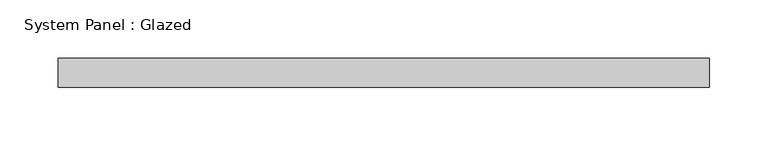
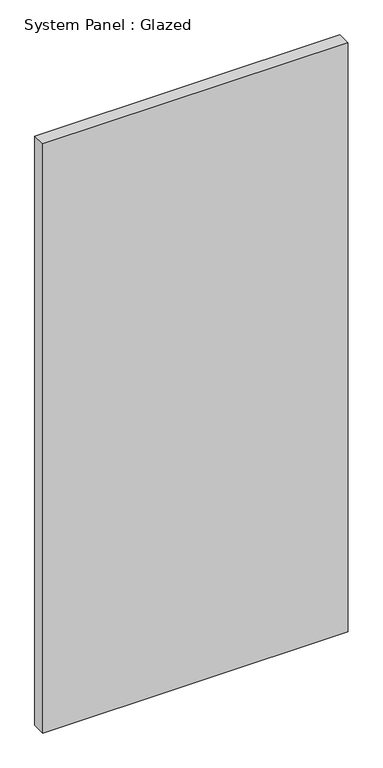
"""IFC4 building model written with IfcOpenShell, lengths in millimetres: plate geometry, System Panel : Glazed."""

from ifc_helpers import new_model, si_unit, origin, origin_with_axes, place, context, project, spatial, polyline, outline, extrude, source, transform, mapped, element, save


def system_panel_glazed_4e5a3e53(model_context):
    return source(origin(), model_context, "Body", "SweptSolid", [
        extrude(outline(polyline([(280.9875, 19.05), (-280.9875, 19.05), (-280.9875, 44.45), (280.9875, 44.45), (280.9875, 19.05)])), origin_with_axes(), (0.0, 0.0, 1.0), 1146.4060005),
    ])


if __name__ == "__main__":
    model = new_model("IFC4")
    model_context = context("Model", 3, world=origin())
    ifc_project = project(units=[si_unit("LENGTHUNIT", "METRE", prefix="MILLI")], contexts=[model_context])
    site = spatial("IfcSite", under=ifc_project)
    building = spatial("IfcBuilding", under=site)
    placement = place(None, origin())
    system_panel_glazed_shape = system_panel_glazed_4e5a3e53(model_context)
    element("IfcPlate", 1, ObjectType="System Panel : Glazed", at=placement, inside=building, context=model_context, shape_type="MappedRepresentation", body=[
        mapped(system_panel_glazed_shape, transform((0.0, 0.0, 0.0), x_axis=(1.0, 0.0, 0.0), y_axis=(0.0, 1.0, 0.0), z_axis=(0.0, 0.0, 1.0))),
    ])
    save(model, "model.ifc")

# Revit data of these elements
# Type "System Panel : Glazed"
#   Construction Type Id = "GSP4R"
#   Analytic Construction = "1/8 in Pilkington single glazing"
#   Visual Light Transmittance = 0.9
#   Solar Heat Gain Coefficient = 0.86
#   Heat Transfer Coefficient (U) = 1.18115 BTU/(h·ft²·°F)
#   Define Thermal Properties by = 1
# Element 1 (IfcPlate, "System Panel : Glazed")
#   Materials on its faces: "Glass"
# Materials
#   "Glass": class "Glass", colour RGB 0 128 192, transparency 0.75, Description = "Soda Lime Glass", Cost = 0
